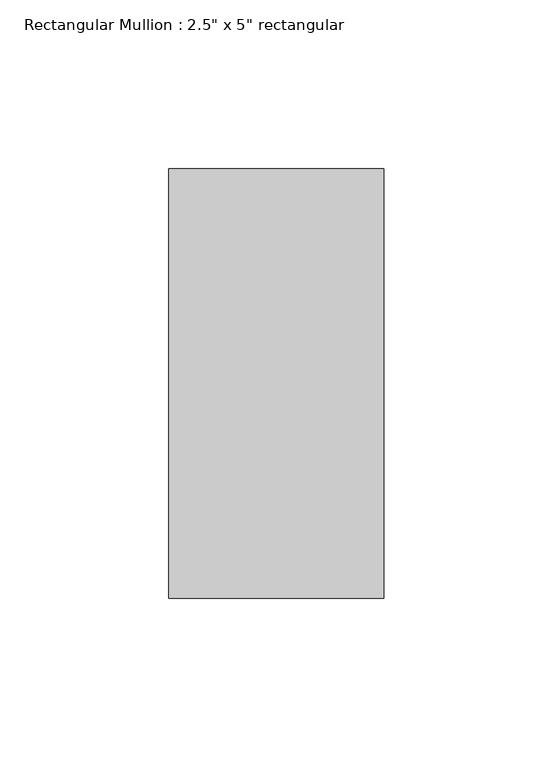
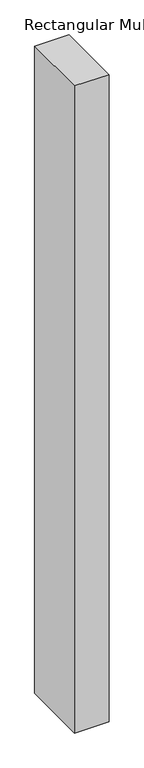
"""IFC4 building model written with IfcOpenShell, lengths in millimetres: member geometry."""

from ifc_helpers import new_model, si_unit, frame, origin, place, context, project, spatial, polyline, outline, extrude, source, transform, mapped, element, save


def member_30a5d983(model_context):
    return source(origin(), model_context, "Body", "SweptSolid", [
        extrude(outline(polyline([(0.0, 63.5), (0.0, -63.5), (-63.5, -63.5), (-63.5, 63.5), (0.0, 63.5)])), frame((0.0, 0.0, -1257.2999998), z_axis=(0.0, 0.0, 1.0), x_axis=(1.0, 0.0, 0.0)), (0.0, 0.0, 1.0), 1257.2999998),
    ])


if __name__ == "__main__":
    model = new_model("IFC4")
    model_context = context("Model", 3, world=origin())
    ifc_project = project(units=[si_unit("LENGTHUNIT", "METRE", prefix="MILLI")], contexts=[model_context])
    site = spatial("IfcSite", under=ifc_project)
    building = spatial("IfcBuilding", under=site)
    placement = place(None, origin())
    member_shape = member_30a5d983(model_context)
    element("IfcMember", 1, ObjectType="Rectangular Mullion : 2.5\" x 5\" rectangular", at=placement, inside=building, context=model_context, shape_type="MappedRepresentation", body=[
        mapped(member_shape, transform((0.0, 0.0, 0.0), x_axis=(1.0, 0.0, 0.0), y_axis=(0.0, 1.0, 0.0), z_axis=(0.0, 0.0, 1.0))),
    ])
    save(model, "model.ifc")

# Revit data of these elements
# Type "Rectangular Mullion : 2.5\" x 5\" rectangular"
#   built-in parameter 1007304 = 0.416667 (stored number, unit not read)
#   built-in parameter 1007301 = 0.104167 (stored number, unit not read)
#   built-in parameter 1007300 = 0.104167 (stored number, unit not read)
# Element 1 (IfcMember, "Rectangular Mullion : 2.5\" x 5\" rectangular")
#   Materials on its faces: "Aluminum"
# Materials
#   "Aluminum": class "Metal", colour RGB 247 247 247, transparency 0, Description = "Aluminum 6061", Cost = 0
